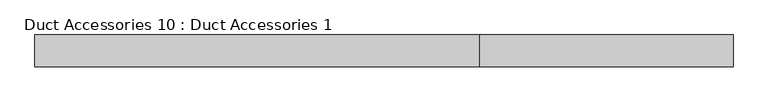
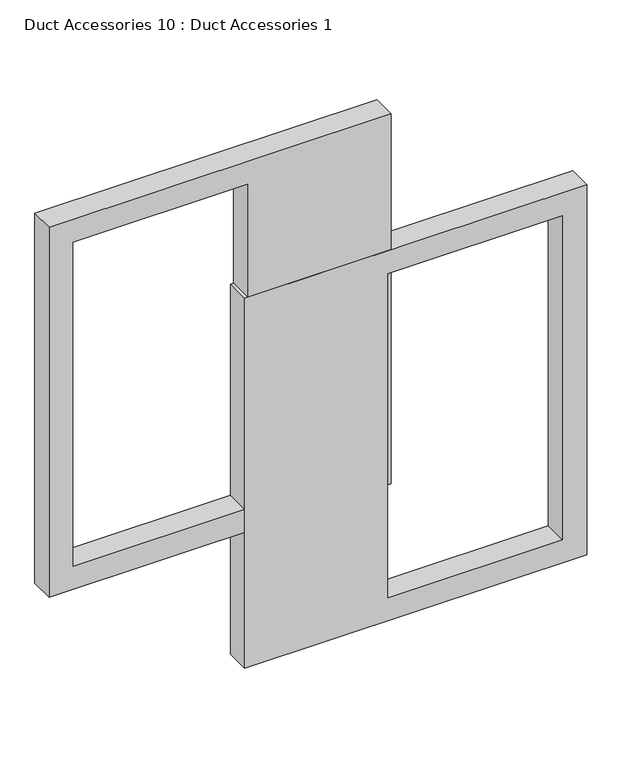
"""IFC4 building model written with IfcOpenShell, lengths in millimetres: damper geometry, Duct Accessories 10 : Duct Accessories 1."""

from ifc_helpers import new_model, si_unit, frame, origin, place, context, project, spatial, polyline, outline, extrude, source, transform, mapped, element, save


def duct_accessories_10_duct_accessories_1_d43a2bea(model_context):
    return source(origin(), model_context, "Body", "SweptSolid", [
        extrude(outline(polyline([(10790.7403114, -12928.36893), (9571.5403114, -12928.36893), (9571.5403114, -11861.56893), (10790.7403114, -11861.56893), (10790.7403114, -12928.36893)]), holes=[polyline([(10714.5403114, -12480.9324751), (10714.5403114, -11937.76893), (9647.7403114, -11937.76893), (9647.7403114, -12480.9324751), (10714.5403114, -12480.9324751)])]), frame((0.0, -447.4934478, 0.0), z_axis=(0.0, 1.0, 0.0), x_axis=(0.0, 0.0, 1.0)), (0.0, 0.0, 1.0), 76.2),
        extrude(outline(polyline([(11238.1767663, -12471.5606701), (11238.1767663, -13538.3606701), (10018.9767663, -13538.3606701), (10018.9767663, -12471.5606701), (11238.1767663, -12471.5606701)]), holes=[polyline([(11161.9767663, -12918.997125), (10095.1767663, -12918.997125), (10095.1767663, -13462.1606701), (11161.9767663, -13462.1606701), (11161.9767663, -12918.997125)])]), frame((0.0, -447.4934478, 0.0), z_axis=(0.0, 1.0, 0.0), x_axis=(0.0, 0.0, 1.0)), (0.0, 0.0, 1.0), 76.2),
    ])


if __name__ == "__main__":
    model = new_model("IFC4")
    model_context = context("Model", 3, world=origin())
    ifc_project = project(units=[si_unit("LENGTHUNIT", "METRE", prefix="MILLI")], contexts=[model_context])
    site = spatial("IfcSite", under=ifc_project)
    building = spatial("IfcBuilding", under=site)
    placement = place(None, origin())
    duct_accessories_10_duct_accessories_1_shape = duct_accessories_10_duct_accessories_1_d43a2bea(model_context)
    element("IfcDamper", 1, ObjectType="Duct Accessories 10 : Duct Accessories 1", at=placement, inside=building, context=model_context, shape_type="MappedRepresentation", body=[
        mapped(duct_accessories_10_duct_accessories_1_shape, transform((0.0, 0.0, 0.0), x_axis=(1.0, 0.0, 0.0), y_axis=(0.0, 1.0, 0.0), z_axis=(0.0, 0.0, 1.0))),
    ])
    save(model, "model.ifc")

# Revit data of these elements
# Element 1 (IfcDamper, "Duct Accessories 10 : Duct Accessories 1")
#   Materials on its faces: "border"
# Materials
#   "border": class "Generic", colour RGB 144 144 144, transparency 0, Cost = 0
